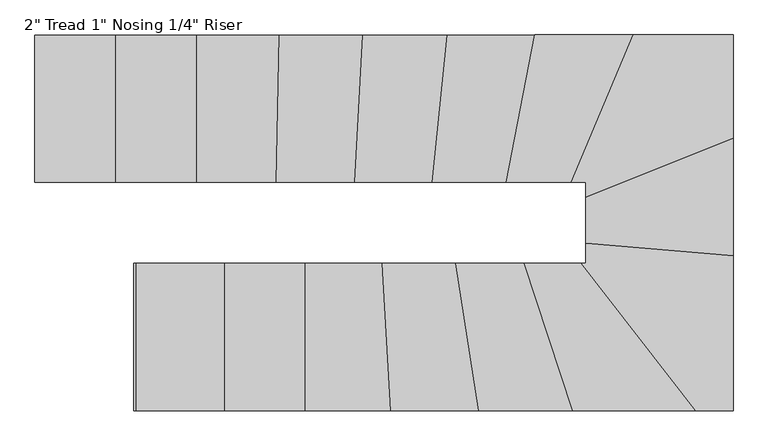
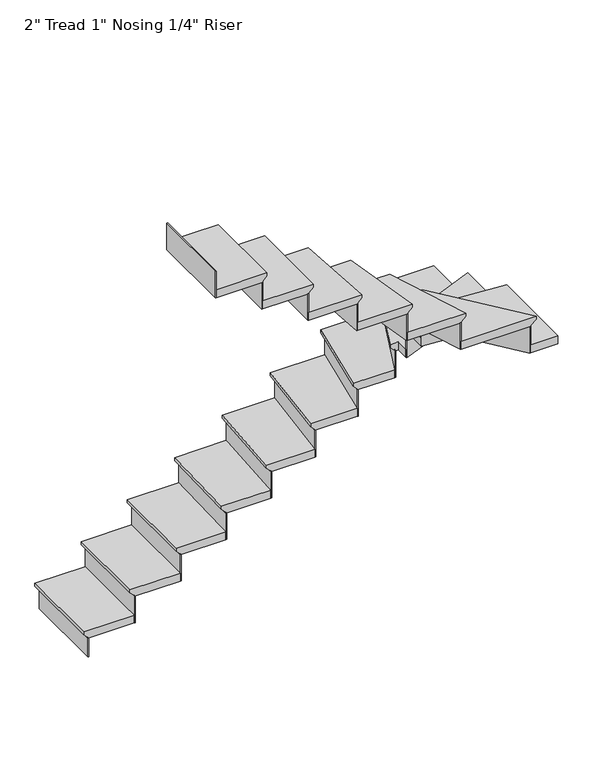
"""IFC4 building model written with IfcOpenShell, lengths in millimetres: stair flight geometry."""

from ifc_helpers import new_model, si_unit, origin, place, context, project, spatial, faceted_brep, source, transform, mapped, element, save


def stair_flight_0d5ba797(model_context):
    return source(origin(), model_context, "Body", "Brep", [
        faceted_brep([(838.4202681, 2693.877558, 6720.4166667), (838.4202681, 2693.877558, 6739.4666667), (838.4202681, 3202.4524989, 6739.4666667), (838.4202681, 3202.4524989, 6720.4166667), (863.8202681, 2693.877558, 6695.0166667), (863.8202681, 3202.4524989, 6695.0166667), (1143.2202681, 2693.877558, 6739.4666667), (1143.2202681, 3202.4524989, 6739.4666667), (863.8202681, 3202.4524989, 6688.6666667), (1143.2202681, 3202.4524989, 6688.6666667), (1143.2202681, 2693.877558, 6688.6666667), (863.8202681, 2693.877558, 6688.6666667)], [[[0, 1, 2, 3]], [[4, 0, 3, 5]], [[2, 1, 6, 7]], [[8, 9, 10, 11]], [[2, 7, 9, 8, 5, 3]], [[8, 11, 4, 5]], [[6, 1, 0, 4, 11, 10]], [[7, 6, 10, 9]]]),
        faceted_brep([(863.8202681, 2693.877558, 6688.6666667), (863.8202681, 2693.877558, 6570.1333333), (870.1702681, 2693.877558, 6570.1333333), (870.1702681, 2693.877558, 6688.6666667), (863.8202681, 3202.4524989, 6688.6666667), (870.1702681, 3202.4524989, 6688.6666667), (870.1702681, 3202.4524989, 6570.1333333), (863.8202681, 3202.4524989, 6570.1333333)], [[[0, 1, 2, 3]], [[4, 5, 6, 7]], [[1, 0, 4, 7]], [[2, 1, 7, 6]], [[3, 2, 6, 5]], [[0, 3, 5, 4]]]),
        faceted_brep([(1143.2202681, 2693.877558, 6858.0), (1143.2202681, 2693.877558, 6688.6666667), (1149.5702681, 2693.877558, 6688.6666667), (1149.5702681, 2693.877558, 6858.0), (1143.2202681, 3202.4524989, 6858.0), (1149.5702681, 3202.4524989, 6858.0), (1149.5702681, 3202.4524989, 6688.6666667), (1143.2202681, 3202.4524989, 6688.6666667)], [[[0, 1, 2, 3]], [[4, 5, 6, 7]], [[1, 0, 4, 7]], [[2, 1, 7, 6]], [[3, 2, 6, 5]], [[0, 3, 5, 4]]]),
        faceted_brep([(1117.8202681, 3202.4524989, 6908.8), (1117.8202681, 2693.877558, 6908.8), (1422.6202681, 2693.877558, 6908.8), (1422.6202681, 3202.4524989, 6908.8), (1143.2202681, 3202.4524989, 6858.0), (1422.6202681, 3202.4524989, 6858.0), (1422.6202681, 2693.877558, 6858.0), (1143.2202681, 2693.877558, 6858.0), (1143.2202681, 3202.4524989, 6864.35), (1117.8202681, 3202.4524989, 6889.75), (1143.2202681, 2693.877558, 6864.35), (1117.8202681, 2693.877558, 6889.75)], [[[0, 1, 2, 3]], [[4, 5, 6, 7]], [[0, 3, 5, 4, 8, 9]], [[4, 7, 10, 8]], [[2, 1, 11, 10, 7, 6]], [[3, 2, 6, 5]], [[11, 1, 0, 9]], [[10, 11, 9, 8]]]),
        faceted_brep([(1422.6202681, 2693.877558, 7027.3333333), (1422.6202681, 2693.877558, 6858.0), (1428.9702681, 2693.877558, 6858.0), (1428.9702681, 2693.877558, 7027.3333333), (1422.6202681, 3202.4524989, 7027.3333333), (1428.9702681, 3202.4524989, 7027.3333333), (1428.9702681, 3202.4524989, 6858.0), (1422.6202681, 3202.4524989, 6858.0)], [[[0, 1, 2, 3]], [[4, 5, 6, 7]], [[1, 0, 4, 7]], [[2, 1, 7, 6]], [[3, 2, 6, 5]], [[0, 3, 5, 4]]]),
        faceted_brep([(1397.2202681, 3202.4524989, 7078.1333333), (1397.2202681, 2693.877558, 7078.1333333), (1696.6553711, 2693.877558, 7078.1333333), (1707.3964935, 3202.4524989, 7078.1333333), (1422.6202681, 3202.4524989, 7027.3333333), (1707.3964935, 3202.4524989, 7027.3333333), (1696.6553711, 2693.877558, 7027.3333333), (1422.6202681, 2693.877558, 7027.3333333), (1422.6202681, 3202.4524989, 7033.6833333), (1397.2202681, 3202.4524989, 7059.0833333), (1422.6202681, 2693.877558, 7033.6833333), (1397.2202681, 2693.877558, 7059.0833333)], [[[0, 1, 2, 3]], [[4, 5, 6, 7]], [[0, 3, 5, 4, 8, 9]], [[4, 7, 10, 8]], [[2, 1, 11, 10, 7, 6]], [[3, 2, 6, 5]], [[11, 1, 0, 9]], [[10, 11, 9, 8]]]),
        faceted_brep([(1696.6553711, 2693.877558, 7196.6666667), (1696.6553711, 2693.877558, 7027.3333333), (1703.0067872, 2693.877558, 7027.3333333), (1703.0067872, 2693.877558, 7196.6666667), (1707.3964935, 3202.4524989, 7196.6666667), (1713.7479096, 3202.4524989, 7196.6666667), (1713.7479096, 3202.4524989, 7027.3333333), (1707.3964935, 3202.4524989, 7027.3333333)], [[[0, 1, 2, 3]], [[4, 5, 6, 7]], [[1, 0, 4, 7]], [[2, 1, 7, 6]], [[3, 2, 6, 5]], [[0, 3, 5, 4]]]),
        faceted_brep([(1681.9908293, 3202.4524989, 7247.4666667), (1671.2497068, 2693.877558, 7247.4666667), (1968.2389719, 2693.877558, 7247.4666667), (1994.6701229, 3202.4524989, 7247.4666667), (1707.3964935, 3202.4524989, 7196.6666667), (1994.6701229, 3202.4524989, 7196.6666667), (1968.2389719, 2693.877558, 7196.6666667), (1696.6553711, 2693.877558, 7196.6666667), (1707.3964935, 3202.4524989, 7203.0166667), (1681.9908293, 3202.4524989, 7228.4166667), (1696.6553711, 2693.877558, 7203.0166667), (1671.2497068, 2693.877558, 7228.4166667)], [[[0, 1, 2, 3]], [[4, 5, 6, 7]], [[0, 3, 5, 4, 8, 9]], [[4, 7, 10, 8]], [[2, 1, 11, 10, 7, 6]], [[3, 2, 6, 5]], [[11, 1, 0, 9]], [[10, 11, 9, 8]]]),
        faceted_brep([(1968.2389719, 2693.877558, 7366.0), (1968.2389719, 2693.877558, 7196.6666667), (1974.5975418, 2693.877558, 7196.6666667), (1974.5975418, 2693.877558, 7366.0), (1994.6701229, 3202.4524989, 7366.0), (2001.0286928, 3202.4524989, 7366.0), (2001.0286928, 3202.4524989, 7196.6666667), (1994.6701229, 3202.4524989, 7196.6666667)], [[[0, 1, 2, 3]], [[4, 5, 6, 7]], [[1, 0, 4, 7]], [[2, 1, 7, 6]], [[3, 2, 6, 5]], [[0, 3, 5, 4]]]),
        faceted_brep([(1969.2358436, 3202.4524989, 7416.8), (1942.8046925, 2693.877558, 7416.8), (2235.1931673, 2693.877558, 7416.8), (2286.7073051, 3202.4524989, 7416.8), (1994.6701229, 3202.4524989, 7366.0), (2286.7073051, 3202.4524989, 7366.0), (2235.1931673, 2693.877558, 7366.0), (1968.2389719, 2693.877558, 7366.0), (1994.6701229, 3202.4524989, 7372.35), (1969.2358436, 3202.4524989, 7397.75), (1968.2389719, 2693.877558, 7372.35), (1942.8046925, 2693.877558, 7397.75)], [[[0, 1, 2, 3]], [[4, 5, 6, 7]], [[0, 3, 5, 4, 8, 9]], [[4, 7, 10, 8]], [[2, 1, 11, 10, 7, 6]], [[3, 2, 6, 5]], [[11, 1, 0, 9]], [[10, 11, 9, 8]]]),
        faceted_brep([(2235.1931673, 2693.877558, 7535.3333333), (2235.1931673, 2693.877558, 7366.0), (2241.5756594, 2693.877558, 7366.0), (2241.5756594, 2693.877558, 7535.3333333), (2286.7073051, 3202.4524989, 7535.3333333), (2293.0897971, 3202.4524989, 7535.3333333), (2293.0897971, 3202.4524989, 7366.0), (2286.7073051, 3202.4524989, 7366.0)], [[[0, 1, 2, 3]], [[4, 5, 6, 7]], [[1, 0, 4, 7]], [[2, 1, 7, 6]], [[3, 2, 6, 5]], [[0, 3, 5, 4]]]),
        faceted_brep([(2261.1773369, 3202.4524989, 7586.1333333), (2209.6631992, 2693.877558, 7586.1333333), (2491.6737127, 2693.877558, 7586.1333333), (2589.7018996, 3202.4524989, 7586.1333333), (2286.7073051, 3202.4524989, 7535.3333333), (2589.7018996, 3202.4524989, 7535.3333333), (2491.6737127, 2693.877558, 7535.3333333), (2235.1931673, 2693.877558, 7535.3333333), (2286.7073051, 3202.4524989, 7541.6833333), (2261.1773369, 3202.4524989, 7567.0833333), (2235.1931673, 2693.877558, 7541.6833333), (2209.6631992, 2693.877558, 7567.0833333)], [[[0, 1, 2, 3]], [[4, 5, 6, 7]], [[0, 3, 5, 4, 8, 9]], [[4, 7, 10, 8]], [[2, 1, 11, 10, 7, 6]], [[3, 2, 6, 5]], [[11, 1, 0, 9]], [[10, 11, 9, 8]]]),
        faceted_brep([(2491.6737127, 2693.877558, 7704.6666667), (2491.6737127, 2693.877558, 7535.3333333), (2498.1405972, 2693.877558, 7535.3333333), (2498.1405972, 2693.877558, 7704.6666667), (2589.7018996, 3202.4524989, 7704.6666667), (2596.1687841, 3202.4524989, 7704.6666667), (2596.1687841, 3202.4524989, 7535.3333333), (2589.7018996, 3202.4524989, 7535.3333333)], [[[0, 1, 2, 3]], [[4, 5, 6, 7]], [[1, 0, 4, 7]], [[2, 1, 7, 6]], [[3, 2, 6, 5]], [[0, 3, 5, 4]]]),
        faceted_brep([(2563.8343615, 3202.4524989, 7755.4666667), (2465.8061746, 2693.877558, 7755.4666667), (2717.082711, 2693.877558, 7755.4666667), (2931.3822032, 3202.4524989, 7755.4666667), (2589.7018996, 3202.4524989, 7704.6666667), (2931.3822032, 3202.4524989, 7704.6666667), (2717.082711, 2693.877558, 7704.6666667), (2491.6737127, 2693.877558, 7704.6666667), (2589.7018996, 3202.4524989, 7711.0166667), (2563.8343615, 3202.4524989, 7736.4166667), (2491.6737127, 2693.877558, 7711.0166667), (2465.8061746, 2693.877558, 7736.4166667)], [[[0, 1, 2, 3]], [[4, 5, 6, 7]], [[0, 3, 5, 4, 8, 9]], [[4, 7, 10, 8]], [[2, 1, 11, 10, 7, 6]], [[3, 2, 6, 5]], [[11, 1, 0, 9]], [[10, 11, 9, 8]]]),
        faceted_brep([(2717.082711, 2693.877558, 7874.0), (2717.082711, 2693.877558, 7704.6666667), (2723.973426, 2693.877558, 7704.6666667), (2723.973426, 2693.877558, 7874.0), (2931.3822032, 3202.4524989, 7874.0), (2938.2729181, 3202.4524989, 7874.0), (2938.2729181, 3202.4524989, 7704.6666667), (2931.3822032, 3202.4524989, 7704.6666667)], [[[0, 1, 2, 3]], [[4, 5, 6, 7]], [[1, 0, 4, 7]], [[2, 1, 7, 6]], [[3, 2, 6, 5]], [[0, 3, 5, 4]]]),
        faceted_brep([(3247.982332, 2818.4435318, 7924.8), (3247.982332, 3202.4524989, 7924.8), (2903.8193433, 3202.4524989, 7924.8), (2689.5198512, 2693.877558, 7924.8), (2739.4073911, 2693.877558, 7924.8), (2739.4073911, 2614.5975609, 7924.8), (3247.982332, 3202.4524989, 7874.0), (3247.982332, 2818.4435318, 7874.0), (2739.4073911, 2614.5975609, 7874.0), (2739.4073911, 2693.877558, 7874.0), (2717.082711, 2693.877558, 7874.0), (2931.3822032, 3202.4524989, 7874.0), (2717.082711, 2693.877558, 7880.35), (2931.3822032, 3202.4524989, 7880.35), (2689.5198512, 2693.877558, 7905.75), (2903.8193433, 3202.4524989, 7905.75)], [[[0, 1, 2, 3, 4, 5]], [[6, 7, 8, 9, 10, 11]], [[1, 0, 7, 6]], [[11, 10, 12, 13]], [[5, 4, 9, 8]], [[0, 5, 8, 7]], [[14, 3, 2, 15]], [[12, 14, 15, 13]], [[4, 3, 14, 12, 10, 9]], [[2, 1, 6, 11, 13, 15]]]),
        faceted_brep([(2739.4073911, 2614.5975609, 8043.3333333), (2739.4073911, 2614.5975609, 7874.0), (2739.4073911, 2607.7564709, 7874.0), (2739.4073911, 2607.7564709, 8043.3333333), (3247.982332, 2818.4435318, 8043.3333333), (3247.982332, 2811.6024418, 8043.3333333), (3247.982332, 2811.6024418, 7874.0), (3247.982332, 2818.4435318, 7874.0)], [[[0, 1, 2, 3]], [[4, 5, 6, 7]], [[1, 0, 4, 7]], [[2, 1, 7, 6]], [[3, 2, 6, 5]], [[0, 3, 5, 4]]]),
        faceted_brep([(3247.982332, 2845.807892, 8094.1333333), (2739.4073911, 2641.9619211, 8094.1333333), (2739.4073911, 2458.7583414, 8094.1333333), (3247.982332, 2415.6151582, 8094.1333333), (3247.982332, 2818.4435318, 8043.3333333), (3247.982332, 2415.6151582, 8043.3333333), (2739.4073911, 2458.7583414, 8043.3333333), (2739.4073911, 2614.5975609, 8043.3333333), (3247.982332, 2818.4435318, 8049.6833333), (3247.982332, 2845.807892, 8075.0833333), (2739.4073911, 2614.5975609, 8049.6833333), (2739.4073911, 2641.9619211, 8075.0833333)], [[[0, 1, 2, 3]], [[4, 5, 6, 7]], [[0, 3, 5, 4, 8, 9]], [[4, 7, 10, 8]], [[2, 1, 11, 10, 7, 6]], [[3, 2, 6, 5]], [[11, 1, 0, 9]], [[10, 11, 9, 8]]]),
        faceted_brep([(2739.4073911, 2458.7583414, 8212.6666667), (2739.4073911, 2458.7583414, 8043.3333333), (2739.4073911, 2452.3855338, 8043.3333333), (2739.4073911, 2452.3855338, 8212.6666667), (3247.982332, 2415.6151582, 8212.6666667), (3247.982332, 2409.2423506, 8212.6666667), (3247.982332, 2409.2423506, 8043.3333333), (3247.982332, 2415.6151582, 8043.3333333)], [[[0, 1, 2, 3]], [[4, 5, 6, 7]], [[1, 0, 4, 7]], [[2, 1, 7, 6]], [[3, 2, 6, 5]], [[0, 3, 5, 4]]]),
        faceted_brep([(3085.5772675, 1905.9026171, 8263.4666667), (3247.982332, 1905.9026171, 8263.4666667), (3247.982332, 2441.1063885, 8263.4666667), (2739.4073911, 2484.2495716, 8263.4666667), (2739.4073911, 2414.477558, 8263.4666667), (2689.4386829, 2414.477558, 8263.4666667), (3247.982332, 1905.9026171, 8212.6666667), (3085.5772675, 1905.9026171, 8212.6666667), (2689.4386829, 2414.477558, 8212.6666667), (2739.4073911, 2414.477558, 8212.6666667), (2739.4073911, 2458.7583414, 8212.6666667), (3247.982332, 2415.6151582, 8212.6666667), (2739.4073911, 2458.7583414, 8219.0166667), (3247.982332, 2415.6151582, 8219.0166667), (2739.4073911, 2484.2495716, 8244.4166667), (3247.982332, 2441.1063885, 8244.4166667)], [[[0, 1, 2, 3, 4, 5]], [[6, 7, 8, 9, 10, 11]], [[1, 0, 7, 6]], [[11, 10, 12, 13]], [[4, 3, 14, 12, 10, 9]], [[5, 4, 9, 8]], [[0, 5, 8, 7]], [[14, 3, 2, 15]], [[12, 14, 15, 13]], [[2, 1, 6, 11, 13, 15]]]),
        faceted_brep([(2689.4386829, 2414.477558, 8382.0), (2689.4386829, 2414.477558, 8212.6666667), (2681.3896615, 2414.477558, 8212.6666667), (2681.3896615, 2414.477558, 8382.0), (3085.5772675, 1905.9026171, 8382.0), (3077.5282461, 1905.9026171, 8382.0), (3077.5282461, 1905.9026171, 8212.6666667), (3085.5772675, 1905.9026171, 8212.6666667)], [[[0, 1, 2, 3]], [[4, 5, 6, 7]], [[1, 0, 4, 7]], [[2, 1, 7, 6]], [[3, 2, 6, 5]], [[0, 3, 5, 4]]]),
        faceted_brep([(3117.7733531, 1905.9026171, 8432.8), (2721.6347685, 2414.477558, 8432.8), (2498.169104, 2414.477558, 8432.8), (2665.6971357, 1905.9026171, 8432.8), (3085.5772675, 1905.9026171, 8382.0), (2665.6971357, 1905.9026171, 8382.0), (2498.169104, 2414.477558, 8382.0), (2689.4386829, 2414.477558, 8382.0), (3085.5772675, 1905.9026171, 8388.35), (3117.7733531, 1905.9026171, 8413.75), (2689.4386829, 2414.477558, 8388.35), (2721.6347685, 2414.477558, 8413.75)], [[[0, 1, 2, 3]], [[4, 5, 6, 7]], [[0, 3, 5, 4, 8, 9]], [[4, 7, 10, 8]], [[2, 1, 11, 10, 7, 6]], [[3, 2, 6, 5]], [[11, 1, 0, 9]], [[10, 11, 9, 8]]]),
        faceted_brep([(2498.169104, 2414.477558, 8551.3333333), (2498.169104, 2414.477558, 8382.0), (2491.4834592, 2414.477558, 8382.0), (2491.4834592, 2414.477558, 8551.3333333), (2665.6971357, 1905.9026171, 8551.3333333), (2659.0114908, 1905.9026171, 8551.3333333), (2659.0114908, 1905.9026171, 8382.0), (2665.6971357, 1905.9026171, 8382.0)], [[[0, 1, 2, 3]], [[4, 5, 6, 7]], [[1, 0, 4, 7]], [[2, 1, 7, 6]], [[3, 2, 6, 5]], [[0, 3, 5, 4]]]),
        faceted_brep([(2692.4397151, 1905.9026171, 8602.1333333), (2524.9116834, 2414.477558, 8602.1333333), (2264.2527614, 2414.477558, 8602.1333333), (2342.8948816, 1905.9026171, 8602.1333333), (2665.6971357, 1905.9026171, 8551.3333333), (2342.8948816, 1905.9026171, 8551.3333333), (2264.2527614, 2414.477558, 8551.3333333), (2498.169104, 2414.477558, 8551.3333333), (2665.6971357, 1905.9026171, 8557.6833333), (2692.4397151, 1905.9026171, 8583.0833333), (2498.169104, 2414.477558, 8557.6833333), (2524.9116834, 2414.477558, 8583.0833333)], [[[0, 1, 2, 3]], [[4, 5, 6, 7]], [[0, 3, 5, 4, 8, 9]], [[4, 7, 10, 8]], [[2, 1, 11, 10, 7, 6]], [[3, 2, 6, 5]], [[11, 1, 0, 9]], [[10, 11, 9, 8]]]),
        faceted_brep([(2264.2527614, 2414.477558, 8720.6666667), (2264.2527614, 2414.477558, 8551.3333333), (2257.827292, 2414.477558, 8551.3333333), (2257.827292, 2414.477558, 8720.6666667), (2342.8948816, 1905.9026171, 8720.6666667), (2336.4694122, 1905.9026171, 8720.6666667), (2336.4694122, 1905.9026171, 8551.3333333), (2342.8948816, 1905.9026171, 8551.3333333)], [[[0, 1, 2, 3]], [[4, 5, 6, 7]], [[1, 0, 4, 7]], [[2, 1, 7, 6]], [[3, 2, 6, 5]], [[0, 3, 5, 4]]]),
        faceted_brep([(2368.5967594, 1905.9026171, 8771.4666667), (2289.9546392, 2414.477558, 8771.4666667), (2009.2587296, 2414.477558, 8771.4666667), (2039.6023306, 1905.9026171, 8771.4666667), (2342.8948816, 1905.9026171, 8720.6666667), (2039.6023306, 1905.9026171, 8720.6666667), (2009.2587296, 2414.477558, 8720.6666667), (2264.2527614, 2414.477558, 8720.6666667), (2342.8948816, 1905.9026171, 8727.0166667), (2368.5967594, 1905.9026171, 8752.4166667), (2264.2527614, 2414.477558, 8727.0166667), (2289.9546392, 2414.477558, 8752.4166667)], [[[0, 1, 2, 3]], [[4, 5, 6, 7]], [[0, 3, 5, 4, 8, 9]], [[4, 7, 10, 8]], [[2, 1, 11, 10, 7, 6]], [[3, 2, 6, 5]], [[11, 1, 0, 9]], [[10, 11, 9, 8]]]),
        faceted_brep([(2009.2587296, 2414.477558, 8890.0), (2009.2587296, 2414.477558, 8720.6666667), (2002.8974373, 2414.477558, 8720.6666667), (2002.8974373, 2414.477558, 8890.0), (2039.6023306, 1905.9026171, 8890.0), (2033.2410383, 1905.9026171, 8890.0), (2033.2410383, 1905.9026171, 8720.6666667), (2039.6023306, 1905.9026171, 8720.6666667)], [[[0, 1, 2, 3]], [[4, 5, 6, 7]], [[1, 0, 4, 7]], [[2, 1, 7, 6]], [[3, 2, 6, 5]], [[0, 3, 5, 4]]]),
        faceted_brep([(2065.0474997, 1905.9026171, 8940.8), (2034.7038988, 2414.477558, 8940.8), (1745.0756993, 2414.477558, 8940.8), (1745.0756993, 1905.9026171, 8940.8), (2039.6023306, 1905.9026171, 8890.0), (1745.0756993, 1905.9026171, 8890.0), (1745.0756993, 2414.477558, 8890.0), (2009.2587296, 2414.477558, 8890.0), (2039.6023306, 1905.9026171, 8896.35), (2065.0474997, 1905.9026171, 8921.75), (2009.2587296, 2414.477558, 8896.35), (2034.7038988, 2414.477558, 8921.75)], [[[0, 1, 2, 3]], [[4, 5, 6, 7]], [[0, 3, 5, 4, 8, 9]], [[4, 7, 10, 8]], [[2, 1, 11, 10, 7, 6]], [[3, 2, 6, 5]], [[11, 1, 0, 9]], [[10, 11, 9, 8]]]),
        faceted_brep([(1745.0756993, 2414.477558, 9059.3333333), (1745.0756993, 2414.477558, 8890.0), (1738.7256993, 2414.477558, 8890.0), (1738.7256993, 2414.477558, 9059.3333333), (1745.0756993, 1905.9026171, 9059.3333333), (1738.7256993, 1905.9026171, 9059.3333333), (1738.7256993, 1905.9026171, 8890.0), (1745.0756993, 1905.9026171, 8890.0)], [[[0, 1, 2, 3]], [[4, 5, 6, 7]], [[1, 0, 4, 7]], [[2, 1, 7, 6]], [[3, 2, 6, 5]], [[0, 3, 5, 4]]]),
        faceted_brep([(1770.4756993, 1905.9026171, 9110.1333333), (1770.4756993, 2414.477558, 9110.1333333), (1465.6756993, 2414.477558, 9110.1333333), (1465.6756993, 1905.9026171, 9110.1333333), (1745.0756993, 1905.9026171, 9059.3333333), (1465.6756993, 1905.9026171, 9059.3333333), (1465.6756993, 2414.477558, 9059.3333333), (1745.0756993, 2414.477558, 9059.3333333), (1745.0756993, 1905.9026171, 9065.6833333), (1770.4756993, 1905.9026171, 9091.0833333), (1745.0756993, 2414.477558, 9065.6833333), (1770.4756993, 2414.477558, 9091.0833333)], [[[0, 1, 2, 3]], [[4, 5, 6, 7]], [[0, 3, 5, 4, 8, 9]], [[4, 7, 10, 8]], [[2, 1, 11, 10, 7, 6]], [[3, 2, 6, 5]], [[11, 1, 0, 9]], [[10, 11, 9, 8]]]),
        faceted_brep([(1465.6756993, 2414.477558, 9228.6666667), (1465.6756993, 2414.477558, 9059.3333333), (1459.3256993, 2414.477558, 9059.3333333), (1459.3256993, 2414.477558, 9228.6666667), (1465.6756993, 1905.9026171, 9228.6666667), (1459.3256993, 1905.9026171, 9228.6666667), (1459.3256993, 1905.9026171, 9059.3333333), (1465.6756993, 1905.9026171, 9059.3333333)], [[[0, 1, 2, 3]], [[4, 5, 6, 7]], [[1, 0, 4, 7]], [[2, 1, 7, 6]], [[3, 2, 6, 5]], [[0, 3, 5, 4]]]),
        faceted_brep([(1186.2756993, 2414.477558, 9398.0), (1186.2756993, 2414.477558, 9228.6666667), (1179.9256993, 2414.477558, 9228.6666667), (1179.9256993, 2414.477558, 9398.0), (1186.2756993, 1905.9026171, 9398.0), (1179.9256993, 1905.9026171, 9398.0), (1179.9256993, 1905.9026171, 9228.6666667), (1186.2756993, 1905.9026171, 9228.6666667)], [[[0, 1, 2, 3]], [[4, 5, 6, 7]], [[1, 0, 4, 7]], [[2, 1, 7, 6]], [[3, 2, 6, 5]], [[0, 3, 5, 4]]]),
        faceted_brep([(1491.0756993, 1905.9026171, 9279.4666667), (1491.0756993, 2414.477558, 9279.4666667), (1186.2756993, 2414.477558, 9279.4666667), (1186.2756993, 1905.9026171, 9279.4666667), (1465.6756993, 1905.9026171, 9228.6666667), (1186.2756993, 1905.9026171, 9228.6666667), (1186.2756993, 2414.477558, 9228.6666667), (1465.6756993, 2414.477558, 9228.6666667), (1465.6756993, 1905.9026171, 9235.0166667), (1491.0756993, 1905.9026171, 9260.4166667), (1465.6756993, 2414.477558, 9235.0166667), (1491.0756993, 2414.477558, 9260.4166667)], [[[0, 1, 2, 3]], [[4, 5, 6, 7]], [[0, 3, 5, 4, 8, 9]], [[4, 7, 10, 8]], [[2, 1, 11, 10, 7, 6]], [[3, 2, 6, 5]], [[11, 1, 0, 9]], [[10, 11, 9, 8]]]),
    ])


if __name__ == "__main__":
    model = new_model("IFC4")
    model_context = context("Model", 3, world=origin())
    ifc_project = project(units=[si_unit("LENGTHUNIT", "METRE", prefix="MILLI")], contexts=[model_context])
    site = spatial("IfcSite", under=ifc_project)
    building = spatial("IfcBuilding", under=site)
    placement = place(None, origin())
    stair_flight_shape = stair_flight_0d5ba797(model_context)
    element("IfcStairFlight", 1, ObjectType="2\" Tread 1\" Nosing 1/4\" Riser", at=placement, inside=building, context=model_context, shape_type="MappedRepresentation", body=[
        mapped(stair_flight_shape, transform((0.0, 0.0, 0.0), x_axis=(1.0, 0.0, 0.0), y_axis=(0.0, 1.0, 0.0), z_axis=(0.0, 0.0, 1.0))),
    ])
    save(model, "model.ifc")
